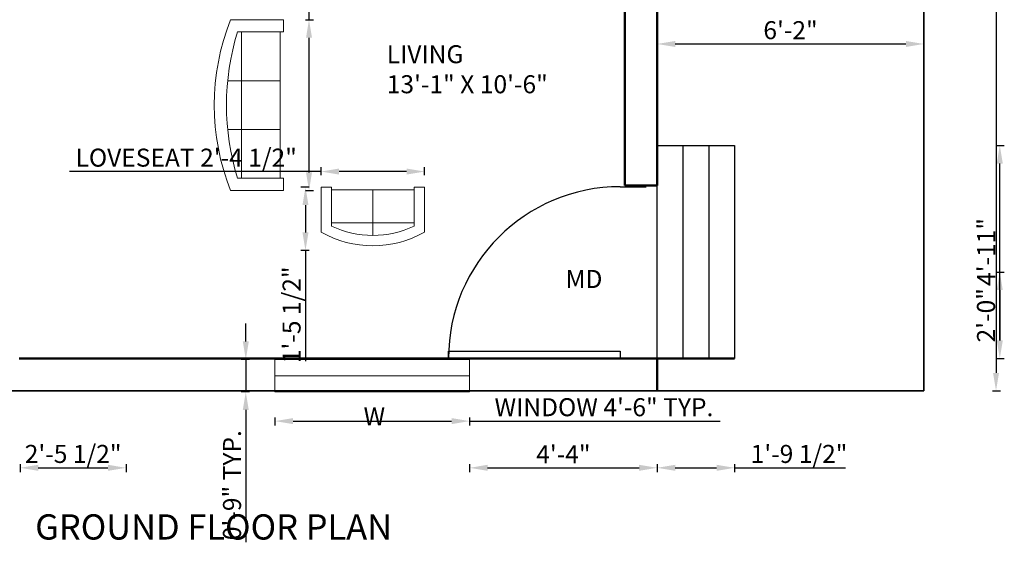
# Model space of a CAD drawing. Units: inches. Extents: x -26 to 423, y -281 to 96.
# Tile 2 of 3: x 147 to 420, y -281 to -136. Entities that reach past the tile are written whole.
import ezdxf

# ---------------------------------------------------------------- set-up
doc = ezdxf.new("R2010")
doc.units = ezdxf.units.IN
doc.header["$PDMODE"] = 35
doc.header["$PDSIZE"] = 5
for name, color, linetype, lineweight in [('A-ANNO-DIMS', 2, 'Continuous', 18), ('A-AREA-IDEN', 7, 'Continuous', 25), ('A-DOOR', 3, 'Continuous', 25), ('A-FLOR-STRS', 7, 'Continuous', 25), ('A-GLAZ', 4, 'Continuous', 18), ('A-WALL', 7, 'Continuous', 50), ('C-PROP', 7, 'Continuous', 35), ('furn', 28, 'Continuous', 18), ('txt', 167, 'Continuous', 18)]:
    doc.layers.add(name, color=color, linetype=linetype, lineweight=lineweight)
doc.styles.get("Standard").update_dxf_attribs({"font": 'arial.ttf'})
doc.dimstyles.new('ISO-25', dxfattribs={"dimtxt": 5, "dimasz": 5, "dimexe": 1.25, "dimexo": 0.625, "dimtad": 1, "dimlunit": 3, "dimtxsty": 'Standard', "dimcen": 2.5, "dimadec": 0, "dimazin": 0, "dimtfac": 1, "dimtmove": 0, "dimatfit": 3, "dimfxl": 1, "dimfxlon": 1, "dimarcsym": 0})

# ---------------------------------------------------------------- blocks, each defined once
blk = doc.blocks.new('*U2')
for p, q in [((0, 0), (0, -6)), ((40, 0), (40, -6))]:
    blk.add_line(p, q)
blk.add_lwpolyline([(0, 0), (0, 40), (1.75, 40), (1.75, 0)], close=True)
blk.add_arc((0, 0), 40, 0, 90)
blk = doc.blocks.new('Sofa - Roundback 7 ft.')
for p, q in [((-12.00002, -32.4421), (-12.00003, -6.5971)), ((11.99997, -32.4421), (11.99998, -6.5971)), ((-36.000027, -34), (-36.000027, -11.4696)), ((-35.999844, -13.3819), (35.9998, -13.3819)), ((35.99998, -34), (35.99998, -11.4696)), ((-36.000027, -32.4421), (35.99998, -32.4421))]:
    blk.add_line(p, q)
for points in [[(-36.000027, -34), (-42.000027, -34), (-42.000027, -8)], [(41.99998, -8), (41.99998, -34), (35.99998, -34)]]:
    blk.add_lwpolyline(points)
for centre, radius, start, end in [((0, -114.25), 114.25, 68.43141, 111.5686), ((-0.00001, -127.1968), 121.1968, 72.72033, 107.2797)]:
    blk.add_arc(centre, radius, start, end)
blk = doc.blocks.new('Sofa - Roundback Loveseat 5 ft.')
for p, q in [((0, -32.44198), (0, -5.99998)), ((-24, -33.99998), (-24, -11.46958)), ((-23.9998, -13.38178), (23.99986, -13.38178)), ((24.00004, -33.99998), (24.00004, -11.46958)), ((-24, -32.44198), (24.00004, -32.44198))]:
    blk.add_line(p, q)
for points in [[(-24, -33.99998), (-30, -33.99998), (-30, -7.99998)], [(30.00004, -7.99998), (30.00004, -33.99998), (24.00004, -33.99998)]]:
    blk.add_lwpolyline(points)
for centre, radius, start, end in [((0, -60.24998), 60.24998, 60.13715, 119.8628), ((0, -61.38438), 55.38444, 64.32083, 115.6792)]:
    blk.add_arc(centre, radius, start, end)
blk = doc.blocks.new('*D11')
at = {"layer": 'A-ANNO-DIMS', "color": 0, "lineweight": -2, "transparency": 16777216}
for p, q in [((323.67, -142.56), (323.67, -141.31)), ((397.67, -142.56), (397.67, -141.31)), ((328.67, -142.56), (392.67, -142.56))]:
    blk.add_line(p, q, dxfattribs=at)
at = {"layer": 'A-ANNO-DIMS', "color": 0, "transparency": 16777216}
for points in [[(328.67, -141.73), (328.67, -143.39), (323.67, -142.56)], [(392.67, -141.73), (392.67, -143.39), (397.67, -142.56)]]:
    blk.add_solid(points, dxfattribs=at)
at = {"layer": 'Defpoints', "color": 0, "transparency": 16777216}
for p in [(323.67, -142.56), (397.67, -142.56), (397.67, -142.56)]:
    blk.add_point(p, dxfattribs=at)
at = {"layer": 'A-ANNO-DIMS', "color": 0, "transparency": 16777216, "insert": (360.67, -139.38), "char_height": 5, "attachment_point": 5}
blk.add_mtext('6\'-2"', dxfattribs=at)
blk = doc.blocks.new('*D13')
at = {"layer": 'A-ANNO-DIMS', "color": 0, "lineweight": -2, "transparency": 16777216}
for p, q in [((416.68, 13.16), (418.93, 13.16)), ((417.68, 8.16), (417.68, -233.84)), ((416.68, -238.84), (418.93, -238.84))]:
    blk.add_line(p, q, dxfattribs=at)
at = {"layer": 'A-ANNO-DIMS', "color": 0, "transparency": 16777216}
for points in [[(416.85, 8.16), (418.51, 8.16), (417.68, 13.16)], [(416.85, -233.84), (418.51, -233.84), (417.68, -238.84)]]:
    blk.add_solid(points, dxfattribs=at)
at = {"layer": 'Defpoints', "color": 0, "transparency": 16777216}
for p in [(397.67, 13.16), (397.67, -238.84), (417.68, -238.84)]:
    blk.add_point(p, dxfattribs=at)
at = {"layer": 'A-ANNO-DIMS', "color": 0, "transparency": 16777216, "insert": (414.55, -112.84), "char_height": 5, "attachment_point": 5, "rotation": 90}
blk.add_mtext("21'", dxfattribs=at)
blk = doc.blocks.new('WINDOW-54IN')
blk.add_line((4.5, 54), (4.5, 0))
blk.add_lwpolyline([(0, 54), (9, 54), (9, 0), (0, 0)], close=True)
blk = doc.blocks.new('*D17')
at = {"layer": 'A-ANNO-DIMS', "color": 0, "lineweight": -2, "transparency": 16777216}
for p, q in [((217.65, -246.21), (217.65, -248.46)), ((222.65, -247.21), (266.65, -247.21)), ((271.65, -246.21), (271.65, -248.46)), ((271.65, -247.21), (341.17, -247.21))]:
    blk.add_line(p, q, dxfattribs=at)
at = {"layer": 'A-ANNO-DIMS', "color": 0, "transparency": 16777216}
for points in [[(222.65, -246.38), (222.65, -248.04), (217.65, -247.21)], [(266.65, -246.38), (266.65, -248.04), (271.65, -247.21)]]:
    blk.add_solid(points, dxfattribs=at)
at = {"layer": 'Defpoints', "color": 0, "transparency": 16777216}
for p in [(217.65, -239.11), (271.65, -239.11), (271.65, -247.21)]:
    blk.add_point(p, dxfattribs=at)
at = {"layer": 'A-ANNO-DIMS', "color": 0, "transparency": 16777216, "insert": (308.91, -244), "char_height": 5, "attachment_point": 5}
blk.add_mtext('WINDOW 4\'-6" TYP.', dxfattribs=at)
blk = doc.blocks.new('*D18')
at = {"layer": 'A-ANNO-DIMS', "color": 0, "lineweight": -2, "transparency": 16777216}
for p, q in [((209.55, -225.11), (209.55, -220.11)), ((210.55, -230.11), (208.3, -230.11)), ((209.55, -230.11), (209.55, -239.11)), ((210.55, -239.11), (208.3, -239.11)), ((209.55, -244.11), (209.55, -280.84))]:
    blk.add_line(p, q, dxfattribs=at)
at = {"layer": 'A-ANNO-DIMS', "color": 0, "transparency": 16777216}
for points in [[(208.72, -225.11), (210.38, -225.11), (209.55, -230.11)], [(208.72, -244.11), (210.38, -244.11), (209.55, -239.11)]]:
    blk.add_solid(points, dxfattribs=at)
at = {"layer": 'Defpoints', "color": 0, "transparency": 16777216}
for p in [(217.65, -230.11), (209.55, -239.11), (217.65, -239.11)]:
    blk.add_point(p, dxfattribs=at)
at = {"layer": 'A-ANNO-DIMS', "color": 0, "transparency": 16777216, "insert": (206.37, -264.98), "char_height": 5, "attachment_point": 5, "rotation": 90}
blk.add_mtext('0\'-9" TYP.', dxfattribs=at)
blk = doc.blocks.new('*D23')
at = {"layer": 'A-ANNO-DIMS', "color": 0, "lineweight": -2, "transparency": 16777216}
for p, q in [((227.09, -135.82), (227.09, -79.81)), ((226.09, -135.82), (228.34, -135.82)), ((227.09, -178.2), (227.09, -140.82)), ((226.09, -183.2), (228.34, -183.2))]:
    blk.add_line(p, q, dxfattribs=at)
at = {"layer": 'A-ANNO-DIMS', "color": 0, "transparency": 16777216}
for points in [[(226.26, -140.82), (227.92, -140.82), (227.09, -135.82)], [(226.26, -178.2), (227.92, -178.2), (227.09, -183.2)]]:
    blk.add_solid(points, dxfattribs=at)
at = {"layer": 'Defpoints', "color": 0, "transparency": 16777216}
for p in [(219.98, -135.82), (227.09, -135.82), (219.98, -183.2)]:
    blk.add_point(p, dxfattribs=at)
at = {"layer": 'A-ANNO-DIMS', "color": 0, "transparency": 16777216, "insert": (223.88, -105.32), "char_height": 5, "attachment_point": 5, "rotation": 90}
blk.add_mtext('SOFA 3\'-11 1/2"', dxfattribs=at)
blk = doc.blocks.new('*D25')
at = {"layer": 'A-ANNO-DIMS', "color": 0, "lineweight": -2, "transparency": 16777216}
for p, q in [((230.42, -178.97), (230.42, -176.72)), ((259.17, -178.97), (259.17, -176.72)), ((230.42, -177.97), (160.63, -177.97)), ((254.17, -177.97), (235.42, -177.97))]:
    blk.add_line(p, q, dxfattribs=at)
at = {"layer": 'A-ANNO-DIMS', "color": 0, "transparency": 16777216}
for points in [[(235.42, -177.13), (235.42, -178.8), (230.42, -177.97)], [(254.17, -177.13), (254.17, -178.8), (259.17, -177.97)]]:
    blk.add_solid(points, dxfattribs=at)
at = {"layer": 'Defpoints', "color": 0, "transparency": 16777216}
for p in [(230.42, -177.97), (230.42, -182.28), (259.17, -182.28)]:
    blk.add_point(p, dxfattribs=at)
at = {"layer": 'A-ANNO-DIMS', "color": 0, "transparency": 16777216, "insert": (193.02, -174.75), "char_height": 5, "attachment_point": 5}
blk.add_mtext('LOVESEAT 2\'-4 1/2"', dxfattribs=at)
blk = doc.blocks.new('*D26')
at = {"layer": 'A-ANNO-DIMS', "color": 0, "lineweight": -2, "transparency": 16777216}
for p, q in [((227.11, -182.28), (224.86, -182.28)), ((226.11, -187.28), (226.11, -194.85)), ((227.11, -199.85), (224.86, -199.85)), ((226.11, -199.85), (226.11, -230.57))]:
    blk.add_line(p, q, dxfattribs=at)
at = {"layer": 'A-ANNO-DIMS', "color": 0, "transparency": 16777216}
for points in [[(225.27, -187.28), (226.94, -187.28), (226.11, -182.28)], [(225.27, -194.85), (226.94, -194.85), (226.11, -199.85)]]:
    blk.add_solid(points, dxfattribs=at)
at = {"layer": 'Defpoints', "color": 0, "transparency": 16777216}
for p in [(230.42, -182.28), (226.11, -199.85), (230.42, -199.85)]:
    blk.add_point(p, dxfattribs=at)
at = {"layer": 'A-ANNO-DIMS', "color": 0, "transparency": 16777216, "insert": (222.9, -217.71), "char_height": 5, "attachment_point": 5, "rotation": 90}
blk.add_mtext('1\'-5 1/2"', dxfattribs=at)
blk = doc.blocks.new('*D36')
at = {"layer": 'A-ANNO-DIMS', "color": 0, "lineweight": -2, "transparency": 16777216}
for p, q in [((271.65, -259.17), (271.65, -261.42)), ((323.67, -259.17), (323.67, -261.42)), ((276.65, -260.17), (318.67, -260.17))]:
    blk.add_line(p, q, dxfattribs=at)
at = {"layer": 'A-ANNO-DIMS', "color": 0, "transparency": 16777216}
for points in [[(276.65, -259.33), (276.65, -261), (271.65, -260.17)], [(318.67, -259.33), (318.67, -261), (323.67, -260.17)]]:
    blk.add_solid(points, dxfattribs=at)
at = {"layer": 'Defpoints', "color": 0, "transparency": 16777216}
for p in [(271.65, -239.11), (323.67, -238.84), (323.67, -260.17)]:
    blk.add_point(p, dxfattribs=at)
at = {"layer": 'A-ANNO-DIMS', "color": 0, "transparency": 16777216, "insert": (297.66, -257.04), "char_height": 5, "attachment_point": 5}
blk.add_mtext('4\'-4"', dxfattribs=at)
blk = doc.blocks.new('*D38')
at = {"layer": 'A-ANNO-DIMS', "color": 0, "lineweight": -2, "transparency": 16777216}
for p, q in [((146.98, -259.17), (146.98, -261.42)), ((176.32, -259.17), (176.32, -261.42)), ((151.98, -260.17), (171.32, -260.17))]:
    blk.add_line(p, q, dxfattribs=at)
at = {"layer": 'A-ANNO-DIMS', "color": 0, "transparency": 16777216}
for points in [[(151.98, -259.33), (151.98, -261), (146.98, -260.17)], [(171.32, -259.33), (171.32, -261), (176.32, -260.17)]]:
    blk.add_solid(points, dxfattribs=at)
at = {"layer": 'Defpoints', "color": 0, "transparency": 16777216}
for p in [(146.98, -50.44), (176.32, -50.84), (176.32, -260.17)]:
    blk.add_point(p, dxfattribs=at)
at = {"layer": 'A-ANNO-DIMS', "color": 0, "transparency": 16777216, "insert": (161.65, -256.96), "char_height": 5, "attachment_point": 5}
blk.add_mtext('2\'-5 1/2"', dxfattribs=at)
blk = doc.blocks.new('*D39')
at = {"layer": 'A-ANNO-DIMS', "color": 0, "lineweight": -2, "transparency": 16777216}
for p, q in [((265.77, 84.21), (265.77, 86.46)), ((270.77, 85.21), (308.46, 85.21)), ((313.46, 84.21), (313.46, 86.46))]:
    blk.add_line(p, q, dxfattribs=at)
at = {"layer": 'A-ANNO-DIMS', "color": 0, "transparency": 16777216}
for points in [[(270.77, 86.05), (270.77, 84.38), (265.77, 85.21)], [(308.46, 86.05), (308.46, 84.38), (313.46, 85.21)]]:
    blk.add_solid(points, dxfattribs=at)
at = {"layer": 'Defpoints', "color": 0, "transparency": 16777216}
for p in [(313.46, 85.21), (265.77, -229.84), (313.46, -229.84)]:
    blk.add_point(p, dxfattribs=at)
at = {"layer": 'A-ANNO-DIMS', "color": 0, "transparency": 16777216, "insert": (289.61, 88.43), "char_height": 5, "attachment_point": 5}
blk.add_mtext('3\'-11 1/2"', dxfattribs=at)
blk = doc.blocks.new('*D44')
at = {"layer": 'A-ANNO-DIMS', "color": 0, "lineweight": -2, "transparency": 16777216}
for p, q in [((323.67, -259.17), (323.67, -261.42)), ((345.17, -259.17), (345.17, -261.42)), ((328.67, -260.17), (340.17, -260.17)), ((345.17, -260.17), (375.89, -260.17))]:
    blk.add_line(p, q, dxfattribs=at)
at = {"layer": 'A-ANNO-DIMS', "color": 0, "transparency": 16777216}
for points in [[(328.67, -259.33), (328.67, -261), (323.67, -260.17)], [(340.17, -259.33), (340.17, -261), (345.17, -260.17)]]:
    blk.add_solid(points, dxfattribs=at)
at = {"layer": 'Defpoints', "color": 0, "transparency": 16777216}
for p in [(323.67, -229.84), (345.17, -229.84), (345.17, -260.17)]:
    blk.add_point(p, dxfattribs=at)
at = {"layer": 'A-ANNO-DIMS', "color": 0, "transparency": 16777216, "insert": (363.03, -256.96), "char_height": 5, "attachment_point": 5}
blk.add_mtext('1\'-9 1/2"', dxfattribs=at)
blk = doc.blocks.new('*D45')
at = {"layer": 'A-ANNO-DIMS', "color": 0, "lineweight": -2, "transparency": 16777216}
for p, q in [((417.73, -170.73), (419.98, -170.73)), ((418.73, -224.84), (418.73, -175.73)), ((417.73, -229.84), (419.98, -229.84))]:
    blk.add_line(p, q, dxfattribs=at)
at = {"layer": 'A-ANNO-DIMS', "color": 0, "transparency": 16777216}
for points in [[(417.89, -175.73), (419.56, -175.73), (418.73, -170.73)], [(417.89, -224.84), (419.56, -224.84), (418.73, -229.84)]]:
    blk.add_solid(points, dxfattribs=at)
at = {"layer": 'Defpoints', "color": 0, "transparency": 16777216}
for p in [(345.17, -170.73), (418.73, -170.73), (345.17, -229.84)]:
    blk.add_point(p, dxfattribs=at)
at = {"layer": 'A-ANNO-DIMS', "color": 0, "transparency": 16777216, "insert": (415.59, -200.29), "char_height": 5, "attachment_point": 5, "rotation": 90}
blk.add_mtext('4\'-11"', dxfattribs=at)
blk = doc.blocks.new('*D55')
at = {"layer": 'A-ANNO-DIMS', "color": 0, "lineweight": -2, "transparency": 16777216}
for p, q in [((417.73, -205.84), (419.98, -205.84)), ((418.73, -210.84), (418.73, -224.84)), ((417.73, -229.84), (419.98, -229.84))]:
    blk.add_line(p, q, dxfattribs=at)
at = {"layer": 'A-ANNO-DIMS', "color": 0, "transparency": 16777216}
for points in [[(417.89, -210.84), (419.56, -210.84), (418.73, -205.84)], [(417.89, -224.84), (419.56, -224.84), (418.73, -229.84)]]:
    blk.add_solid(points, dxfattribs=at)
at = {"layer": 'Defpoints', "color": 0, "transparency": 16777216}
for p in [(79.39, -205.84), (79.39, -229.84), (418.73, -229.84)]:
    blk.add_point(p, dxfattribs=at)
at = {"layer": 'A-ANNO-DIMS', "color": 0, "transparency": 16777216, "insert": (415.55, -217.84), "char_height": 5, "attachment_point": 5, "rotation": 90}
blk.add_mtext('2\'-0"', dxfattribs=at)

msp = doc.modelspace()

# ---------------------------------------------------------------- linework, layer by layer
at = {"layer": 'A-FLOR-STRS'}
for p, q in [((323.673, -170.73), (345.168, -170.73)), ((323.673, -229.842), (323.673, -170.73)), ((330.838, -170.73), (330.838, -229.842)), ((338.003, -170.73), (338.003, -229.842)), ((345.168, -170.73), (345.168, -229.842)), ((345.168, -229.842), (323.673, -229.842))]:
    msp.add_line(p, q, dxfattribs=at)
at = {"layer": 'A-WALL'}
for p, q in [((323.673, -181.842), (323.673, 13.158)), ((314.673, -181.842), (314.673, -102.842)), ((323.673, -181.842), (314.673, -181.842)), ((198.673, -229.842), (146.673, -229.842)), ((202.673, -229.842), (198.673, -229.842)), ((345.168, -229.842), (202.673, -229.842)), ((323.673, -229.842), (323.673, -238.842))]:
    msp.add_line(p, q, dxfattribs=at)
at = {"layer": 'C-PROP'}
for p, q in [((397.673, 13.158), (397.673, -238.842)), ((397.673, -238.842), (1.673, -238.842))]:
    msp.add_line(p, q, dxfattribs=at)

# ---------------------------------------------------------------- block references
at = {"layer": 'A-DOOR', "xscale": 1.192034194377611, "yscale": 1.192034194377611, "zscale": 1.192034194377611, "rotation": 90}
msp.add_blockref('*U2', (313.455, -229.842), dxfattribs=at)
at = {"layer": 'A-GLAZ', "rotation": 270}
msp.add_blockref('WINDOW-54IN', (217.649, -230.112), dxfattribs=at)
at = {"layer": 'furn'}
for name, p, xscale, yscale, zscale, rotation in [('Sofa - Roundback 7 ft.', (200.806, -159.515), 0.5640572462292086, 0.5640572462292086, 0.5640572462292086, 90), ('Sofa - Roundback Loveseat 5 ft.', (244.792, -198.569), 0.4791470912556123, 0.4791470912556123, 0.4791470912556123, 180)]:
    msp.add_blockref(name, p, dxfattribs=dict(at, xscale=xscale, yscale=yscale, zscale=zscale, rotation=rotation))

# ---------------------------------------------------------------- texts
at = {"layer": 'A-AREA-IDEN', "insert": (248.655, -142.903), "char_height": 5, "attachment_point": 1}
msp.add_mtext_dynamic_manual_height_columns('LIVING\\P13\'-1" X 10\'-6"', width=45.89436, gutter_width=12.5, heights=[0], dxfattribs=at)
at = {"layer": 'txt', "attachment_point": 1}
for s, width, insert, char_height in [('MD', 18.84569, (298.252, -205.274), 5), ('W', 10.55725, (242.219, -243.351), 5), ('GROUND FLOOR PLAN', 249.0726, (151.115, -273.078), 7)]:
    msp.add_mtext_dynamic_manual_height_columns(s, width=width, gutter_width=12.5, heights=[0], dxfattribs=dict(at, insert=insert, char_height=char_height))

# ---------------------------------------------------------------- dimensions: what is measured, and where the dimension line sits
at = {"layer": 'A-ANNO-DIMS'}
for base, p1, p2, override, picture, middle in [((313.455, 85.213), (265.774, -229.842), (313.455, -229.842), {"dimdec": 1, "dimlfac": 1, "dimrnd": 0, "dimzin": 1, "dimdsep": 46, "dimlunit": 4, "dimfrac": 2}, '*D39', (289.614, 88.425)), ((176.324, -260.167), (146.978, -50.44), (176.324, -50.842), {"dimdec": 1, "dimlfac": 1, "dimrnd": 0, "dimzin": 1, "dimdsep": 46, "dimlunit": 4, "dimfrac": 2}, '*D38', (161.651, -256.956)), ((397.673, -142.56), (323.673, -142.56), (397.673, -142.56), {"dimclrd": 0, "dimclre": 0, "dimclrt": 0}, '*D11', (360.673, -139.382)), ((345.168, -260.167), (323.673, -229.842), (345.168, -229.842), {"dimdec": 1, "dimlfac": 1, "dimrnd": 0, "dimzin": 1, "dimdsep": 46, "dimlunit": 4, "dimfrac": 2}, '*D44', (363.029, -256.956)), ((323.673, -260.167), (271.649, -239.112), (323.673, -238.842), {"dimdec": 1, "dimlfac": 1, "dimrnd": 0, "dimzin": 1, "dimdsep": 46, "dimlunit": 4, "dimfrac": 2}, '*D36', (297.661, -257.042))]:
    dim = msp.add_linear_dim(base=base, p1=p1, p2=p2, dimstyle='ISO-25', override=override, dxfattribs=at)
    dim.commit()
    dim.dimension.update_dxf_attribs({"geometry": picture, "text_midpoint": middle})
for base, p1, p2, angle, override, picture, middle in [((417.681, -238.842), (397.673, 13.158), (397.673, -238.842), 90, {"dimclrd": 0, "dimclre": 0, "dimclrt": 0}, '*D13', (414.546, -112.842)), ((418.728, -170.73), (345.168, -229.842), (345.168, -170.73), 90, {"dimdec": 1, "dimlfac": 1, "dimrnd": 0, "dimzin": 1, "dimdsep": 46, "dimlunit": 4, "dimfrac": 2}, '*D45', (415.592, -200.286)), ((226.106, -199.846), (230.418, -182.278), (230.418, -199.846), 270, {"dimdec": 1, "dimlfac": 1, "dimrnd": 0, "dimzin": 1, "dimdsep": 46, "dimlunit": 4, "dimfrac": 2}, '*D26', (222.895, -217.707)), ((418.728, -229.842), (79.395, -205.842), (79.395, -229.842), 90, {"dimdec": 1, "dimlfac": 1, "dimrnd": 0, "dimzin": 1, "dimdsep": 46, "dimlunit": 4, "dimfrac": 2}, '*D55', (415.55, -217.842))]:
    dim = msp.add_linear_dim(base=base, p1=p1, p2=p2, angle=angle, dimstyle='ISO-25', override=override, dxfattribs=at)
    dim.commit()
    dim.dimension.update_dxf_attribs({"geometry": picture, "text_midpoint": middle})
for base, p1, p2, angle, text, picture, middle in [((227.091, -135.824), (219.984, -183.205), (219.984, -135.824), 90, 'SOFA <>', '*D23', (223.877, -105.319)), ((230.418, -177.965), (259.167, -182.278), (230.418, -182.278), 180, 'LOVESEAT <>', '*D25', (193.023, -174.753)), ((209.549, -239.112), (217.649, -230.112), (217.649, -239.112), 270, '<> TYP.', '*D18', (206.371, -264.975))]:
    dim = msp.add_linear_dim(base=base, p1=p1, p2=p2, angle=angle, text=text, dimstyle='ISO-25', override={"dimdec": 1, "dimlfac": 1, "dimrnd": 0, "dimzin": 1, "dimdsep": 46, "dimlunit": 4, "dimfrac": 2}, dxfattribs=at)
    dim.commit()
    dim.dimension.update_dxf_attribs({"geometry": picture, "text_midpoint": middle})
dim = msp.add_linear_dim(base=(271.649, -247.212), p1=(217.649, -239.112), p2=(271.649, -239.112), text='WINDOW <> TYP.', dimstyle='ISO-25', override={"dimdec": 1, "dimlfac": 1, "dimrnd": 0, "dimzin": 1, "dimdsep": 46, "dimlunit": 4, "dimfrac": 2}, dxfattribs=at)
dim.commit()
dim.dimension.update_dxf_attribs({"geometry": '*D17', "text_midpoint": (308.91, -244)})

doc.saveas('drawing.dxf')
